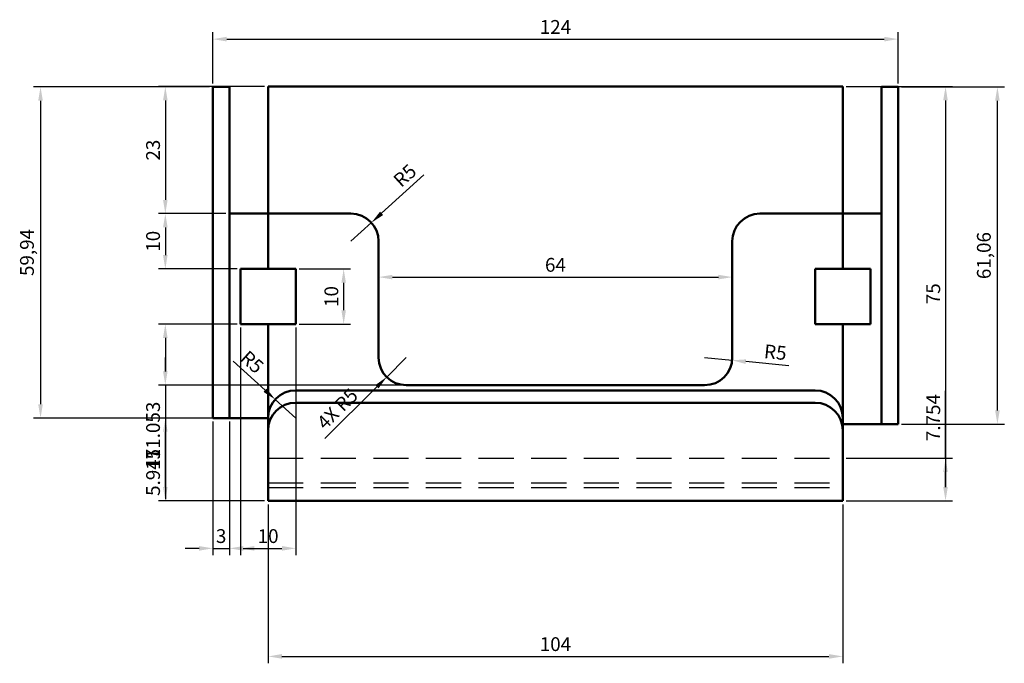
# Model space of a CAD drawing. Units: millimetres. Extents: x 1154 to 1562, y 1225 to 1481.
# Tile 1 of 4: x 1154 to 1332, y 1241 to 1357. Entities that reach past the tile are written whole.
import ezdxf

# ---------------------------------------------------------------- set-up
doc = ezdxf.new("R2010")
doc.units = ezdxf.units.MM
doc.linetypes.add('HIDDEN', pattern=[9.525, 6.35, -3.175])
for name, color, linetype, lineweight in [('M-DIMS', 2, 'Continuous', 25), ('M-HIDN', 4, 'HIDDEN', 25), ('M-OUTL', 7, 'Continuous', 50)]:
    doc.layers.add(name, color=color, linetype=linetype, lineweight=lineweight)
doc.styles.get("Standard").update_dxf_attribs({"font": 'arial.ttf'})
doc.dimstyles.new('ISO-25', dxfattribs={"dimtxt": 2.5, "dimasz": 2.5, "dimexe": 1.25, "dimexo": 0.625, "dimtad": 1, "dimtxsty": 'Standard', "dimcen": 2.5, "dimadec": 0, "dimazin": 0, "dimtfac": 1, "dimtmove": 0, "dimatfit": 3, "dimfxl": 1, "dimarcsym": 0})

# ---------------------------------------------------------------- blocks, each defined once
blk = doc.blocks.new('*D26')
at = {"layer": 'Defpoints', "color": 0, "transparency": 16777216}
for p in [(1199.05, 1270.29), (1303.05, 1270.29), (1303.05, 1242.13)]:
    blk.add_point(p, dxfattribs=at)
at = {"layer": 'M-DIMS', "color": 0, "lineweight": -2, "transparency": 16777216}
for p, q in [((1199.05, 1269.66), (1199.05, 1240.88)), ((1303.05, 1269.66), (1303.05, 1240.88)), ((1201.55, 1242.13), (1300.55, 1242.13))]:
    blk.add_line(p, q, dxfattribs=at)
at = {"layer": 'M-DIMS', "color": 0, "transparency": 16777216}
for points in [[(1201.55, 1242.55), (1201.55, 1241.71), (1199.05, 1242.13)], [(1300.55, 1242.55), (1300.55, 1241.71), (1303.05, 1242.13)]]:
    blk.add_solid(points, dxfattribs=at)
at = {"layer": 'M-DIMS', "color": 0, "transparency": 16777216, "insert": (1251.05, 1244.03), "char_height": 2.5, "attachment_point": 5}
blk.add_mtext('104', dxfattribs=at)
blk = doc.blocks.new('*D27')
at = {"layer": 'Defpoints', "color": 0, "transparency": 16777216}
for p in [(1189.05, 1345.23), (1157.86, 1285.29), (1189.05, 1285.29)]:
    blk.add_point(p, dxfattribs=at)
at = {"layer": 'M-DIMS', "color": 0, "lineweight": -2, "transparency": 16777216}
for p, q in [((1188.42, 1345.23), (1156.61, 1345.23)), ((1157.86, 1342.73), (1157.86, 1287.79)), ((1188.42, 1285.29), (1156.61, 1285.29))]:
    blk.add_line(p, q, dxfattribs=at)
at = {"layer": 'M-DIMS', "color": 0, "transparency": 16777216}
for points in [[(1157.44, 1342.73), (1158.28, 1342.73), (1157.86, 1345.23)], [(1157.44, 1287.79), (1158.28, 1287.79), (1157.86, 1285.29)]]:
    blk.add_solid(points, dxfattribs=at)
at = {"layer": 'M-DIMS', "color": 0, "transparency": 16777216, "insert": (1155.73, 1315.26), "char_height": 2.5, "attachment_point": 5, "rotation": 90}
blk.add_mtext('59,94', dxfattribs=at)
blk = doc.blocks.new('*D28')
at = {"layer": 'Defpoints', "color": 0, "transparency": 16777216}
for p in [(1204.05, 1312.29), (1204.05, 1302.29), (1212.72, 1302.29)]:
    blk.add_point(p, dxfattribs=at)
at = {"layer": 'M-DIMS', "color": 0, "lineweight": -2, "transparency": 16777216}
for p, q in [((1204.67, 1312.29), (1213.97, 1312.29)), ((1212.72, 1309.79), (1212.72, 1304.79)), ((1204.67, 1302.29), (1213.97, 1302.29))]:
    blk.add_line(p, q, dxfattribs=at)
at = {"layer": 'M-DIMS', "color": 0, "transparency": 16777216}
for points in [[(1212.31, 1309.79), (1213.14, 1309.79), (1212.72, 1312.29)], [(1212.31, 1304.79), (1213.14, 1304.79), (1212.72, 1302.29)]]:
    blk.add_solid(points, dxfattribs=at)
at = {"layer": 'M-DIMS', "color": 0, "transparency": 16777216, "insert": (1210.82, 1307.29), "char_height": 2.5, "attachment_point": 5, "rotation": 90}
blk.add_mtext('10', dxfattribs=at)
blk = doc.blocks.new('*D29')
at = {"layer": 'Defpoints', "color": 0, "transparency": 16777216}
for p in [(1200.34, 1288.65), (1204.05, 1285.29)]:
    blk.add_point(p, dxfattribs=at)
at = {"layer": 'M-DIMS', "color": 0, "lineweight": -2, "transparency": 16777216}
for p, q in [((1192.71, 1295.56), (1198.49, 1290.32)), ((1204.05, 1285.29), (1200.34, 1288.65))]:
    blk.add_line(p, q, dxfattribs=at)
at = {"layer": 'M-DIMS', "color": 0, "transparency": 16777216}
blk.add_solid([(1198.77, 1290.63), (1198.21, 1290.02), (1200.34, 1288.65)], dxfattribs=at)
at = {"layer": 'M-DIMS', "color": 0, "transparency": 16777216, "insert": (1195.95, 1295.19), "char_height": 2.5, "attachment_point": 5, "rotation": 317.8212}
blk.add_mtext('R5', dxfattribs=at)
blk = doc.blocks.new('*D30')
at = {"layer": 'Defpoints', "color": 0, "transparency": 16777216}
for p in [(1217.74, 1320.66), (1214.05, 1317.29)]:
    blk.add_point(p, dxfattribs=at)
at = {"layer": 'M-DIMS', "color": 0, "lineweight": -2, "transparency": 16777216}
for p, q in [((1227.25, 1329.34), (1219.59, 1322.35)), ((1214.05, 1317.29), (1217.74, 1320.66))]:
    blk.add_line(p, q, dxfattribs=at)
at = {"layer": 'M-DIMS', "color": 0, "transparency": 16777216}
blk.add_solid([(1219.31, 1322.65), (1219.87, 1322.04), (1217.74, 1320.66)], dxfattribs=at)
at = {"layer": 'M-DIMS', "color": 0, "transparency": 16777216, "insert": (1224.02, 1328.95), "char_height": 2.5, "attachment_point": 5, "rotation": 42.3905}
blk.add_mtext('R5', dxfattribs=at)
blk = doc.blocks.new('*D31')
at = {"layer": 'Defpoints', "color": 0, "transparency": 16777216}
for p in [(1278.05, 1296.24), (1283.02, 1295.74)]:
    blk.add_point(p, dxfattribs=at)
at = {"layer": 'M-DIMS', "color": 0, "lineweight": -2, "transparency": 16777216}
for p, q in [((1278.05, 1296.24), (1283.02, 1295.74)), ((1293.27, 1294.73), (1285.51, 1295.5))]:
    blk.add_line(p, q, dxfattribs=at)
at = {"layer": 'M-DIMS', "color": 0, "transparency": 16777216}
blk.add_solid([(1285.55, 1295.91), (1285.47, 1295.08), (1283.02, 1295.74)], dxfattribs=at)
at = {"layer": 'M-DIMS', "color": 0, "transparency": 16777216, "insert": (1290.82, 1296.88), "char_height": 2.5, "attachment_point": 5, "rotation": 354.344}
blk.add_mtext('R5', dxfattribs=at)
blk = doc.blocks.new('*D60')
at = {"layer": 'Defpoints', "color": 0, "transparency": 16777216}
for p in [(1313.05, 1345.23), (1331.04, 1345.23), (1313.05, 1284.17)]:
    blk.add_point(p, dxfattribs=at)
at = {"layer": 'M-DIMS', "color": 0, "lineweight": -2, "transparency": 16777216}
for p, q in [((1313.67, 1345.23), (1332.29, 1345.23)), ((1331.04, 1286.67), (1331.04, 1342.73)), ((1313.67, 1284.17), (1332.29, 1284.17))]:
    blk.add_line(p, q, dxfattribs=at)
at = {"layer": 'M-DIMS', "color": 0, "transparency": 16777216}
for points in [[(1330.62, 1342.73), (1331.45, 1342.73), (1331.04, 1345.23)], [(1330.62, 1286.67), (1331.45, 1286.67), (1331.04, 1284.17)]]:
    blk.add_solid(points, dxfattribs=at)
at = {"layer": 'M-DIMS', "color": 0, "transparency": 16777216, "insert": (1328.91, 1314.7), "char_height": 2.5, "attachment_point": 5, "rotation": 90}
blk.add_mtext('61,06', dxfattribs=at)
blk = doc.blocks.new('*D61')
at = {"layer": 'Defpoints', "color": 0, "transparency": 16777216}
for p in [(1283.05, 1310.8), (1219.05, 1306.76), (1283.05, 1306.76)]:
    blk.add_point(p, dxfattribs=at)
at = {"layer": 'M-DIMS', "color": 0, "lineweight": -2, "transparency": 16777216}
for p, q in [((1219.05, 1307.39), (1219.05, 1312.05)), ((1283.05, 1307.39), (1283.05, 1312.05)), ((1221.55, 1310.8), (1280.55, 1310.8))]:
    blk.add_line(p, q, dxfattribs=at)
at = {"layer": 'M-DIMS', "color": 0, "transparency": 16777216}
for points in [[(1221.55, 1311.22), (1221.55, 1310.39), (1219.05, 1310.8)], [(1280.55, 1311.22), (1280.55, 1310.39), (1283.05, 1310.8)]]:
    blk.add_solid(points, dxfattribs=at)
at = {"layer": 'M-DIMS', "color": 0, "transparency": 16777216, "insert": (1251.05, 1312.7), "char_height": 2.5, "attachment_point": 5}
blk.add_mtext('64', dxfattribs=at)
blk = doc.blocks.new('*D77')
at = {"layer": 'Defpoints', "color": 0, "transparency": 16777216}
for p in [(1313.05, 1353.89), (1189.05, 1345.23), (1313.05, 1345.23)]:
    blk.add_point(p, dxfattribs=at)
at = {"layer": 'M-DIMS', "color": 0, "lineweight": -2, "transparency": 16777216}
for p, q in [((1189.05, 1345.85), (1189.05, 1355.14)), ((1313.05, 1345.85), (1313.05, 1355.14)), ((1191.55, 1353.89), (1310.55, 1353.89))]:
    blk.add_line(p, q, dxfattribs=at)
at = {"layer": 'M-DIMS', "color": 0, "transparency": 16777216}
for points in [[(1191.55, 1354.31), (1191.55, 1353.47), (1189.05, 1353.89)], [(1310.55, 1354.31), (1310.55, 1353.47), (1313.05, 1353.89)]]:
    blk.add_solid(points, dxfattribs=at)
at = {"layer": 'M-DIMS', "color": 0, "transparency": 16777216, "insert": (1251.05, 1355.77), "char_height": 2.5, "attachment_point": 5}
blk.add_mtext('124', dxfattribs=at)
blk = doc.blocks.new('*D78')
at = {"layer": 'Defpoints', "color": 0, "transparency": 16777216}
for p in [(1303.05, 1345.29), (1303.05, 1270.29), (1321.65, 1270.29)]:
    blk.add_point(p, dxfattribs=at)
at = {"layer": 'M-DIMS', "color": 0, "lineweight": -2, "transparency": 16777216}
for p, q in [((1303.67, 1345.29), (1322.9, 1345.29)), ((1321.65, 1342.79), (1321.65, 1272.79)), ((1303.67, 1270.29), (1322.9, 1270.29))]:
    blk.add_line(p, q, dxfattribs=at)
at = {"layer": 'M-DIMS', "color": 0, "transparency": 16777216}
for points in [[(1321.23, 1342.79), (1322.06, 1342.79), (1321.65, 1345.29)], [(1321.23, 1272.79), (1322.06, 1272.79), (1321.65, 1270.29)]]:
    blk.add_solid(points, dxfattribs=at)
at = {"layer": 'M-DIMS', "color": 0, "transparency": 16777216, "insert": (1319.75, 1307.79), "char_height": 2.5, "attachment_point": 5, "rotation": 90}
blk.add_mtext('75', dxfattribs=at)
blk = doc.blocks.new('*D79')
at = {"layer": 'Defpoints', "color": 0, "transparency": 16777216}
for p in [(1189.05, 1285.29), (1192.05, 1285.29), (1192.05, 1261.69)]:
    blk.add_point(p, dxfattribs=at)
at = {"layer": 'M-DIMS', "color": 0, "lineweight": -2, "transparency": 16777216}
for p, q in [((1189.05, 1284.66), (1189.05, 1260.44)), ((1192.05, 1284.66), (1192.05, 1260.44)), ((1186.55, 1261.69), (1184.05, 1261.69)), ((1189.05, 1261.69), (1192.05, 1261.69)), ((1194.55, 1261.69), (1197.05, 1261.69))]:
    blk.add_line(p, q, dxfattribs=at)
at = {"layer": 'M-DIMS', "color": 0, "transparency": 16777216}
for points in [[(1186.55, 1262.11), (1186.55, 1261.27), (1189.05, 1261.69)], [(1194.55, 1262.11), (1194.55, 1261.27), (1192.05, 1261.69)]]:
    blk.add_solid(points, dxfattribs=at)
at = {"layer": 'M-DIMS', "color": 0, "transparency": 16777216, "insert": (1190.55, 1263.59), "char_height": 2.5, "attachment_point": 5}
blk.add_mtext('3', dxfattribs=at)
blk = doc.blocks.new('*D80')
at = {"layer": 'Defpoints', "color": 0, "transparency": 16777216}
for p in [(1194.05, 1302.29), (1204.05, 1302.29), (1204.05, 1261.69)]:
    blk.add_point(p, dxfattribs=at)
at = {"layer": 'M-DIMS', "color": 0, "lineweight": -2, "transparency": 16777216}
for p, q in [((1194.05, 1301.66), (1194.05, 1260.44)), ((1204.05, 1301.66), (1204.05, 1260.44)), ((1196.55, 1261.69), (1201.55, 1261.69))]:
    blk.add_line(p, q, dxfattribs=at)
at = {"layer": 'M-DIMS', "color": 0, "transparency": 16777216}
for points in [[(1196.55, 1262.11), (1196.55, 1261.27), (1194.05, 1261.69)], [(1201.55, 1262.11), (1201.55, 1261.27), (1204.05, 1261.69)]]:
    blk.add_solid(points, dxfattribs=at)
at = {"layer": 'M-DIMS', "color": 0, "transparency": 16777216, "insert": (1199.05, 1263.59), "char_height": 2.5, "attachment_point": 5}
blk.add_mtext('10', dxfattribs=at)
blk = doc.blocks.new('*D81')
at = {"layer": 'Defpoints', "color": 0, "transparency": 16777216}
for p in [(1199.05, 1345.29), (1180.45, 1322.29), (1192.05, 1322.29)]:
    blk.add_point(p, dxfattribs=at)
at = {"layer": 'M-DIMS', "color": 0, "lineweight": -2, "transparency": 16777216}
for p, q in [((1198.42, 1345.29), (1179.2, 1345.29)), ((1180.45, 1342.79), (1180.45, 1324.79)), ((1191.42, 1322.29), (1179.2, 1322.29))]:
    blk.add_line(p, q, dxfattribs=at)
at = {"layer": 'M-DIMS', "color": 0, "transparency": 16777216}
for points in [[(1180.03, 1342.79), (1180.86, 1342.79), (1180.45, 1345.29)], [(1180.03, 1324.79), (1180.86, 1324.79), (1180.45, 1322.29)]]:
    blk.add_solid(points, dxfattribs=at)
at = {"layer": 'M-DIMS', "color": 0, "transparency": 16777216, "insert": (1178.55, 1333.79), "char_height": 2.5, "attachment_point": 5, "rotation": 90}
blk.add_mtext('23', dxfattribs=at)
blk = doc.blocks.new('*D82')
at = {"layer": 'Defpoints', "color": 0, "transparency": 16777216}
for p in [(1192.05, 1322.29), (1180.45, 1312.29), (1194.05, 1312.29)]:
    blk.add_point(p, dxfattribs=at)
at = {"layer": 'M-DIMS', "color": 0, "lineweight": -2, "transparency": 16777216}
for p, q in [((1191.42, 1322.29), (1179.2, 1322.29)), ((1180.45, 1319.79), (1180.45, 1314.79)), ((1193.42, 1312.29), (1179.2, 1312.29))]:
    blk.add_line(p, q, dxfattribs=at)
at = {"layer": 'M-DIMS', "color": 0, "transparency": 16777216}
for points in [[(1180.03, 1319.79), (1180.86, 1319.79), (1180.45, 1322.29)], [(1180.03, 1314.79), (1180.86, 1314.79), (1180.45, 1312.29)]]:
    blk.add_solid(points, dxfattribs=at)
at = {"layer": 'M-DIMS', "color": 0, "transparency": 16777216, "insert": (1178.55, 1317.29), "char_height": 2.5, "attachment_point": 5, "rotation": 90}
blk.add_mtext('10', dxfattribs=at)
blk = doc.blocks.new('*D83')
at = {"layer": 'Defpoints', "color": 0, "transparency": 16777216}
for p in [(1194.05, 1302.29), (1180.45, 1291.24), (1224.05, 1291.24)]:
    blk.add_point(p, dxfattribs=at)
at = {"layer": 'M-DIMS', "color": 0, "lineweight": -2, "transparency": 16777216}
for p, q in [((1193.42, 1302.29), (1179.2, 1302.29)), ((1180.45, 1299.79), (1180.45, 1293.74)), ((1223.42, 1291.24), (1179.2, 1291.24)), ((1180.45, 1291.24), (1180.45, 1277.34))]:
    blk.add_line(p, q, dxfattribs=at)
at = {"layer": 'M-DIMS', "color": 0, "transparency": 16777216}
for points in [[(1180.03, 1299.79), (1180.86, 1299.79), (1180.45, 1302.29)], [(1180.03, 1293.74), (1180.86, 1293.74), (1180.45, 1291.24)]]:
    blk.add_solid(points, dxfattribs=at)
at = {"layer": 'M-DIMS', "color": 0, "transparency": 16777216, "insert": (1178.55, 1283.04), "char_height": 2.5, "attachment_point": 5, "rotation": 90}
blk.add_mtext('11.053', dxfattribs=at)
blk = doc.blocks.new('*D84')
at = {"layer": 'Defpoints', "color": 0, "transparency": 16777216}
for p in [(1224.05, 1291.24), (1180.45, 1285.29), (1192.05, 1285.29)]:
    blk.add_point(p, dxfattribs=at)
at = {"layer": 'M-DIMS', "color": 0, "lineweight": -2, "transparency": 16777216}
for p, q in [((1180.45, 1293.74), (1180.45, 1296.24)), ((1223.42, 1291.24), (1179.2, 1291.24)), ((1180.45, 1291.24), (1180.45, 1285.29)), ((1191.42, 1285.29), (1179.2, 1285.29)), ((1180.45, 1282.79), (1180.45, 1270.6))]:
    blk.add_line(p, q, dxfattribs=at)
at = {"layer": 'M-DIMS', "color": 0, "transparency": 16777216}
for points in [[(1180.03, 1293.74), (1180.86, 1293.74), (1180.45, 1291.24)], [(1180.03, 1282.79), (1180.86, 1282.79), (1180.45, 1285.29)]]:
    blk.add_solid(points, dxfattribs=at)
at = {"layer": 'M-DIMS', "color": 0, "transparency": 16777216, "insert": (1178.55, 1275.45), "char_height": 2.5, "attachment_point": 5, "rotation": 90}
blk.add_mtext('5.947', dxfattribs=at)
blk = doc.blocks.new('*D85')
at = {"layer": 'Defpoints', "color": 0, "transparency": 16777216}
for p in [(1180.45, 1285.29), (1199.05, 1285.29), (1199.05, 1270.29)]:
    blk.add_point(p, dxfattribs=at)
at = {"layer": 'M-DIMS', "color": 0, "lineweight": -2, "transparency": 16777216}
for p, q in [((1198.42, 1285.29), (1179.2, 1285.29)), ((1180.45, 1272.79), (1180.45, 1282.79)), ((1198.42, 1270.29), (1179.2, 1270.29))]:
    blk.add_line(p, q, dxfattribs=at)
at = {"layer": 'M-DIMS', "color": 0, "transparency": 16777216}
for points in [[(1180.03, 1282.79), (1180.86, 1282.79), (1180.45, 1285.29)], [(1180.03, 1272.79), (1180.86, 1272.79), (1180.45, 1270.29)]]:
    blk.add_solid(points, dxfattribs=at)
at = {"layer": 'M-DIMS', "color": 0, "transparency": 16777216, "insert": (1178.55, 1277.79), "char_height": 2.5, "attachment_point": 5, "rotation": 90}
blk.add_mtext('15', dxfattribs=at)
blk = doc.blocks.new('*D86')
at = {"layer": 'Defpoints', "color": 0, "transparency": 16777216}
for p in [(1303.05, 1278.04), (1321.65, 1278.04), (1303.05, 1270.29)]:
    blk.add_point(p, dxfattribs=at)
at = {"layer": 'M-DIMS', "color": 0, "lineweight": -2, "transparency": 16777216}
for p, q in [((1321.65, 1278.04), (1321.65, 1290.2)), ((1303.67, 1278.04), (1322.9, 1278.04)), ((1321.65, 1272.79), (1321.65, 1275.54)), ((1303.67, 1270.29), (1322.9, 1270.29))]:
    blk.add_line(p, q, dxfattribs=at)
at = {"layer": 'M-DIMS', "color": 0, "transparency": 16777216}
for points in [[(1321.23, 1275.54), (1322.06, 1275.54), (1321.65, 1278.04)], [(1321.23, 1272.79), (1322.06, 1272.79), (1321.65, 1270.29)]]:
    blk.add_solid(points, dxfattribs=at)
at = {"layer": 'M-DIMS', "color": 0, "transparency": 16777216, "insert": (1319.75, 1285.37), "char_height": 2.5, "attachment_point": 5, "rotation": 90}
blk.add_mtext('7.754', dxfattribs=at)
blk = doc.blocks.new('*D100')
at = {"layer": 'Defpoints', "color": 0, "transparency": 16777216}
for p in [(1224.05, 1296.24), (1220.51, 1292.71)]:
    blk.add_point(p, dxfattribs=at)
at = {"layer": 'M-DIMS', "color": 0, "lineweight": -2, "transparency": 16777216}
for p, q in [((1224.05, 1296.24), (1220.51, 1292.71)), ((1209.33, 1281.57), (1218.74, 1290.94))]:
    blk.add_line(p, q, dxfattribs=at)
at = {"layer": 'M-DIMS', "color": 0, "transparency": 16777216}
blk.add_solid([(1218.44, 1291.24), (1219.03, 1290.65), (1220.51, 1292.71)], dxfattribs=at)
at = {"layer": 'M-DIMS', "color": 0, "transparency": 16777216, "insert": (1211.81, 1286.72), "char_height": 2.5, "attachment_point": 5, "rotation": 44.9026}
blk.add_mtext('4X R5', dxfattribs=at)

msp = doc.modelspace()

# ---------------------------------------------------------------- linework, layer by layer
at = {"layer": 'M-HIDN'}
for p, q in [((1199.0479, 1278.0428), (1303.0479, 1278.0428)), ((1199.0479, 1273.5426), (1303.0479, 1273.5426)), ((1199.0479, 1272.6815), (1303.0479, 1272.6815))]:
    msp.add_line(p, q, dxfattribs=at)
at = {"layer": 'M-OUTL'}
for p, q in [((1189.0479, 1285.2887), (1189.0479, 1345.2296)), ((1189.0479, 1345.2296), (1192.0479, 1345.2296)), ((1192.0479, 1345.2296), (1192.0479, 1285.2887)), ((1303.0479, 1345.2887), (1199.0479, 1345.2887)), ((1199.0479, 1345.2887), (1199.0479, 1335.2887)), ((1303.0479, 1335.2887), (1303.0479, 1345.2887)), ((1313.0479, 1345.2296), (1310.0479, 1345.2296)), ((1310.0479, 1345.2296), (1310.0479, 1284.1704)), ((1313.0479, 1284.1704), (1313.0479, 1345.2296)), ((1199.0479, 1335.2887), (1199.0479, 1322.2887)), ((1303.0479, 1335.2887), (1303.0479, 1322.2887)), ((1214.0479, 1322.2887), (1192.0479, 1322.2887)), ((1199.0479, 1322.2887), (1199.0479, 1312.2887)), ((1288.0479, 1322.2887), (1310.0479, 1322.2887)), ((1303.0479, 1322.2887), (1303.0479, 1312.2887)), ((1219.0479, 1296.2358), (1219.0479, 1317.2887)), ((1283.0479, 1296.2358), (1283.0479, 1317.2887)), ((1199.0479, 1312.2887), (1194.0479, 1312.2887)), ((1194.0479, 1312.2887), (1194.0479, 1302.2887)), ((1204.0479, 1312.2887), (1199.0479, 1312.2887)), ((1204.0479, 1302.2887), (1204.0479, 1312.2887)), ((1303.0479, 1312.2887), (1298.0479, 1312.2887)), ((1298.0479, 1312.2887), (1298.0479, 1302.2887)), ((1308.0479, 1312.2887), (1303.0479, 1312.2887)), ((1308.0479, 1302.2887), (1308.0479, 1312.2887)), ((1194.0479, 1302.2887), (1204.0479, 1302.2887)), ((1199.0479, 1302.2887), (1199.0479, 1283.0522)), ((1298.0479, 1302.2887), (1308.0479, 1302.2887)), ((1303.0479, 1302.2887), (1303.0479, 1284.1704)), ((1204.0479, 1290.2887), (1298.0479, 1290.2887)), ((1224.0479, 1291.2358), (1278.0479, 1291.2358)), ((1204.0479, 1288.0522), (1298.0479, 1288.0522)), ((1199.0479, 1285.2887), (1189.0479, 1285.2887)), ((1199.0479, 1285.2887), (1199.0479, 1270.2887)), ((1303.0479, 1285.2887), (1303.0479, 1283.0522)), ((1199.0479, 1270.2887), (1199.0479, 1283.0522)), ((1303.0479, 1284.1704), (1313.0479, 1284.1704)), ((1303.0479, 1270.2887), (1303.0479, 1283.0522)), ((1199.0479, 1270.2887), (1303.0479, 1270.2887)), ((1199.0479, 1270.2887), (1219.0479, 1270.2887)), ((1303.0479, 1270.2887), (1283.0479, 1270.2887))]:
    msp.add_line(p, q, dxfattribs=at)
for centre, start, end in [((1214.0479, 1317.2887), 0, 90), ((1288.0479, 1317.2887), 90, 180), ((1224.0479, 1296.2358), 180, 270), ((1278.0479, 1296.2358), 270, 0), ((1204.0479, 1285.2887), 90, 180), ((1298.0479, 1285.2887), 0, 90), ((1204.0479, 1283.0522), 90, 180), ((1298.0479, 1283.0522), 0, 90)]:
    msp.add_arc(centre, 5, start, end, dxfattribs=at)

# ---------------------------------------------------------------- dimensions: what is measured, and where the dimension line sits
at = {"layer": 'M-DIMS'}
for base, p1, p2, override, picture, middle in [((1313.0479, 1353.8887), (1189.0479, 1345.2296), (1313.0479, 1345.2296), {"dimdec": 0, "dimlfac": 1, "dimrnd": 0, "dimzin": 0, "dimdsep": 46, "dimlunit": 2}, '*D77', (1251.0479, 1355.7688)), ((1283.0479, 1310.8022), (1219.0479, 1306.7623), (1283.0479, 1306.7623), {"dimclrd": 0, "dimclre": 0, "dimclrt": 0}, '*D61', (1251.0479, 1312.7036)), ((1204.0479, 1261.6887), (1194.0479, 1302.2887), (1204.0479, 1302.2887), {"dimdec": 0, "dimlfac": 1, "dimrnd": 0, "dimzin": 0, "dimdsep": 46, "dimlunit": 2}, '*D80', (1199.0479, 1263.5901)), ((1192.0479, 1261.6887), (1189.0479, 1285.2887), (1192.0479, 1285.2887), {"dimdec": 0, "dimlfac": 1, "dimrnd": 0, "dimzin": 0, "dimdsep": 46, "dimlunit": 2}, '*D79', (1190.5479, 1263.591)), ((1303.0479, 1242.1288), (1199.0479, 1270.2887), (1303.0479, 1270.2887), {"dimclrd": 0, "dimclre": 0, "dimclrt": 0}, '*D26', (1251.0479, 1244.0302))]:
    dim = msp.add_linear_dim(base=base, p1=p1, p2=p2, dimstyle='ISO-25', override=override, dxfattribs=at)
    dim.commit()
    dim.dimension.update_dxf_attribs({"geometry": picture, "text_midpoint": middle})
for base, p1, p2, override, picture, middle in [((1157.8586, 1285.2887), (1189.0479, 1345.2296), (1189.0479, 1285.2887), {"dimclrd": 0, "dimclre": 0, "dimclrt": 0}, '*D27', (1155.7312, 1315.2591)), ((1180.4479, 1322.2887), (1199.0479, 1345.2887), (1192.0479, 1322.2887), {"dimdec": 0, "dimlfac": 1, "dimrnd": 0, "dimzin": 0, "dimdsep": 46, "dimlunit": 2}, '*D81', (1178.5456, 1333.7887)), ((1321.6479, 1270.2887), (1303.0479, 1345.2887), (1303.0479, 1270.2887), {"dimdec": 0, "dimlfac": 1, "dimrnd": 0, "dimzin": 0, "dimdsep": 46, "dimlunit": 2}, '*D78', (1319.7516, 1307.7887)), ((1331.0354, 1345.2296), (1313.0479, 1284.1704), (1313.0479, 1345.2296), {"dimclrd": 0, "dimclre": 0, "dimclrt": 0}, '*D60', (1328.908, 1314.7)), ((1180.4479, 1312.2887), (1192.0479, 1322.2887), (1194.0479, 1312.2887), {"dimdec": 0, "dimlfac": 1, "dimrnd": 0, "dimzin": 0, "dimdsep": 46, "dimlunit": 2}, '*D82', (1178.5464, 1317.2887)), ((1212.7242, 1302.2887), (1204.0479, 1312.2887), (1204.0479, 1302.2887), {"dimclrd": 0, "dimclre": 0, "dimclrt": 0}, '*D28', (1210.8228, 1307.2887)), ((1180.4479, 1291.2358), (1194.0479, 1302.2887), (1224.0479, 1291.2358), {"dimdec": 3, "dimlfac": 1, "dimrnd": 0, "dimzin": 0, "dimdsep": 46, "dimlunit": 2}, '*D83', (1178.5456, 1283.0392)), ((1180.4479, 1285.2887), (1224.0479, 1291.2358), (1192.0479, 1285.2887), {"dimdec": 3, "dimlfac": 1, "dimrnd": 0, "dimzin": 0, "dimdsep": 46, "dimlunit": 2}, '*D84', (1178.5464, 1275.4456)), ((1321.6479, 1278.0428), (1303.0479, 1270.2887), (1303.0479, 1278.0428), {"dimdec": 3, "dimlfac": 1, "dimrnd": 0, "dimzin": 0, "dimdsep": 46, "dimlunit": 2}, '*D86', (1319.7516, 1285.3706)), ((1180.4479, 1285.2887), (1199.0479, 1270.2887), (1199.0479, 1285.2887), {"dimdec": 0, "dimlfac": 1, "dimrnd": 0, "dimzin": 0, "dimdsep": 46, "dimlunit": 2}, '*D85', (1178.5464, 1277.7887))]:
    dim = msp.add_linear_dim(base=base, p1=p1, p2=p2, angle=90, dimstyle='ISO-25', override=override, dxfattribs=at)
    dim.commit()
    dim.dimension.update_dxf_attribs({"geometry": picture, "text_midpoint": middle})
dim = msp.add_radius_dim(center=(1214.0479, 1317.2887), mpoint=(1217.7407, 1320.6596), dimstyle='ISO-25', override={"dimclrd": 0, "dimclre": 0, "dimclrt": 0}, dxfattribs=at)
dim.commit()
dim.dimension.update_dxf_attribs({"geometry": '*D30', "text_midpoint": (1225.2935, 1327.554), "dimtype": 164})
for center, mpoint, picture, middle in [((1204.0479, 1285.2887), (1200.3426, 1288.6459), '*D29', (1195.9468, 1295.1878)), ((1278.0479, 1296.2358), (1283.0235, 1295.743), '*D31', (1290.8232, 1296.8762))]:
    dim = msp.add_radius_dim(center=center, mpoint=mpoint, dimstyle='ISO-25', override={"dimclrd": 0, "dimclre": 0, "dimclrt": 0}, dxfattribs=at)
    dim.commit()
    dim.dimension.update_dxf_attribs({"geometry": picture, "text_midpoint": middle})
dim = msp.add_radius_dim(center=(1224.0479, 1296.2358), mpoint=(1220.5063, 1292.7063), text='4X <>', dimstyle='ISO-25', override={"dimdec": 0, "dimlfac": 1, "dimrnd": 0, "dimzin": 0, "dimdsep": 46, "dimlunit": 2}, dxfattribs=at)
dim.commit()
dim.dimension.update_dxf_attribs({"geometry": '*D100', "text_midpoint": (1211.811, 1286.7178)})

doc.saveas('drawing.dxf')
